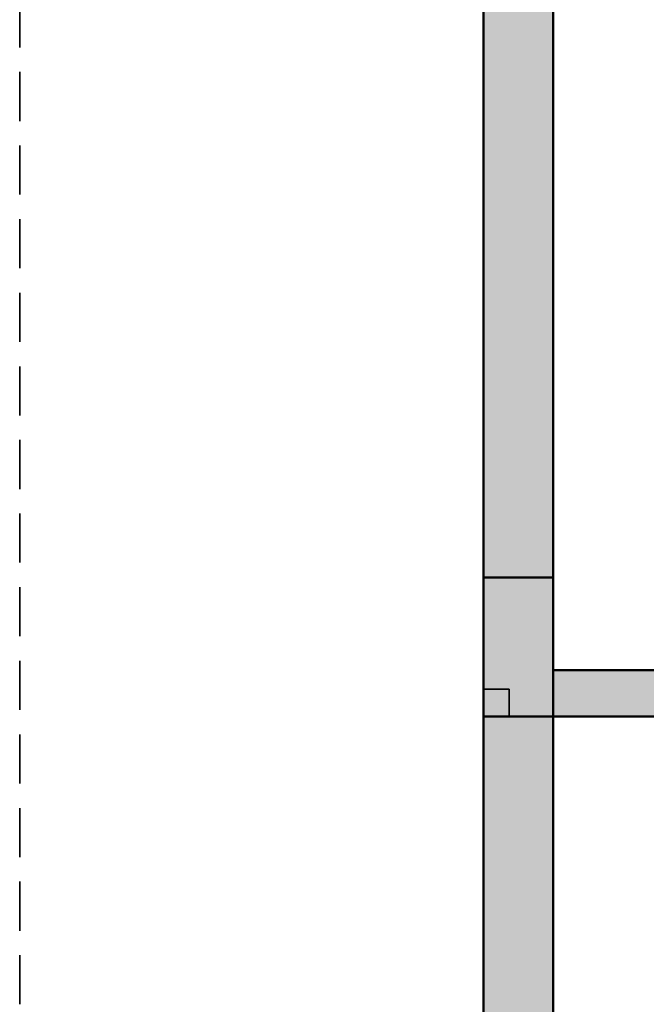
# Model space of a CAD drawing. Units: inches. Extents: x -7 to 1228, y -146 to 1091.
# Tile 43 of 88: x 0 to 81, y 531 to 658. Entities that reach past the tile are written whole.
import ezdxf

# ---------------------------------------------------------------- set-up
doc = ezdxf.new("R2010")
doc.units = ezdxf.units.IN
doc.linetypes.add('DASHED2', pattern=[9.525, 6.35, -3.175])
for name, color, linetype, lineweight in [('A-COLS', 6, 'Continuous', 35), ('A-WALL', 7, 'Continuous', 50), ('A-WALL-PATT', 251, 'Continuous', 13), ('C-PROP', 1, 'DASHED2', 35)]:
    doc.layers.add(name, color=color, linetype=linetype, lineweight=lineweight)

msp = doc.modelspace()

# ---------------------------------------------------------------- hatches: boundary and pattern name
at = {"layer": 'A-COLS'}
h = msp.add_hatch(color=256, dxfattribs=at)
h.dxf.hatch_style = 1
h.paths.add_polyline_path([(69, 586), (60, 586), (60, 571.55), (63.29, 571.55), (63.29, 568), (69, 568)])
h = msp.add_hatch(color=256, dxfattribs=at)
h.dxf.hatch_style = 1
h.paths.add_polyline_path([(63.29, 571.55), (60, 571.55), (60, 568), (63.29, 568)])
at = {"layer": 'A-WALL-PATT'}
h = msp.add_hatch(color=256, dxfattribs=at)
h.dxf.hatch_style = 1
h.paths.add_polyline_path([(69, 568), (60, 568), (60, 493), (63.29, 493), (69, 493)])
h.paths.add_polyline_path([(69, 662.41), (60, 662.41), (60, 586), (69, 586)], flags=17)
h.paths.add_polyline_path([(69, 723), (184, 723), (184, 734), (179, 734), (179, 728), (69, 728), (69, 741.62), (60, 741.62), (60, 698.41), (69, 698.41)], flags=17)
h.paths.add_polyline_path([(69, 782), (231, 782), (231, 728), (231, 723), (231, 586), (236, 586), (236, 787), (69, 787), (69, 800.13), (60, 800.13), (60, 765.62), (69, 765.62)])
h.paths.add_polyline_path([(184, 842), (189, 842), (189, 848), (173, 848), (173, 842), (179, 842), (179, 787), (184, 787)])
h.paths.add_polyline_path([(118.22, 69), (69, 69), (69, 60), (118.22, 60)])
h.paths.add_polyline_path([(227, 69), (154.22, 69), (154.22, 60), (227, 60)])
h.paths.add_polyline_path([(236, 60), (232.71, 60), (227, 60), (227, 36), (236, 36)])
h.paths.add_polyline_path([(389, 60), (380, 60), (380, 36), (389, 36)])
h.paths.add_polyline_path([(384, 181), (380, 181), (380, 115), (380, 78), (384, 78)])
h.paths.add_polyline_path([(380, 115), (334.55, 115), (334.55, 109), (380, 109)])
h.paths.add_polyline_path([(274.55, 115), (236, 115), (236, 201), (232.71, 201), (231, 201), (231, 78), (236, 78), (236, 109), (274.55, 109)])
h.paths.add_polyline_path([(69, 123), (60, 123), (60, 78), (69, 78)])
h.paths.add_polyline_path([(69, 201), (60, 201), (60, 159), (69, 159)])
h.paths.add_polyline_path([(143, 219), (69, 219), (69, 213), (143, 213)], flags=17)
h.paths.add_polyline_path([(189, 219), (184, 219), (184, 274), (231, 274), (231, 219), (236, 219), (236, 279), (184, 279), (184, 297), (179, 297), (179, 279), (69, 279), (69, 290.91), (60, 290.91), (60, 262.18), (69, 262.18), (69, 274), (179, 274), (179, 219), (173, 219), (173, 213), (189, 213)])
h.paths.add_polyline_path([(69, 238.18), (60, 238.18), (60, 219), (69, 219)], flags=17)
h.paths.add_polyline_path([(69, 333), (60, 333), (60, 314.91), (69, 314.91), (69, 316.96)])
h.paths.add_polyline_path([(190, 338), (184, 338), (69, 338), (69, 333), (179, 333), (179, 327), (184, 327), (184, 333.02), (190, 333.05)])
h.paths.add_polyline_path([(69, 386.81), (60, 386.81), (60, 351), (69, 351)])
h.paths.add_polyline_path([(69, 475), (60, 475), (60, 422.81), (69, 422.81)])
h.paths.add_polyline_path([(236, 475), (231, 475), (231, 351.24), (236, 351.24)])
h.paths.add_polyline_path([(384, 475), (380, 475), (380, 362), (384, 362)])
h.paths.add_polyline_path([(547, 307), (439, 307), (439, 356), (445, 356), (445, 362), (433, 362), (433, 307), (380, 307), (380, 244), (380, 241), (384, 241), (384, 301), (433, 301), (433, 277), (439, 277), (439, 301), (547, 301)])
h.paths.add_polyline_path([(547, 241), (439, 241), (439, 247), (433, 247), (433, 235), (547, 235)])
h.paths.add_polyline_path([(450, 69), (440.29, 69), (424.89, 69), (389, 69), (389, 60), (450, 60)])
h.paths.add_polyline_path([(547, 69), (486, 69), (486, 60), (547, 60)])
h.paths.add_polyline_path([(556, 148.27), (547, 148.27), (547, 78), (556, 78)])
h.paths.add_polyline_path([(556, 223), (547, 223), (547, 195), (547, 184.27), (556, 184.27)])
h.paths.add_polyline_path([(556, 311.19), (547, 311.19), (547, 273.08), (556, 273.08)])
h.paths.add_polyline_path([(556, 344), (552.71, 344), (547, 344), (547, 335.19), (556, 335.19)])
h.paths.add_polyline_path([(556, 249.08), (547, 249.08), (547, 241), (556, 241)])
h.paths.add_polyline_path([(547, 362), (475, 362), (475, 356), (547, 356)], flags=0)
h.paths.add_polyline_path([(556, 399.62), (547, 399.62), (547, 362), (556, 362)])
h.paths.add_polyline_path([(556, 475), (547, 475), (547, 435.62), (556, 435.62)])
h.paths.add_polyline_path([(547, 493), (389, 493), (389, 487), (547, 487)])
h.paths.add_polyline_path([(380, 493), (278, 493), (278, 487), (380, 487)])
h.paths.add_polyline_path([(227, 493), (69, 493), (69, 487), (227, 487)])
h.paths.add_polyline_path([(643, 122.44), (634, 122.44), (634, 78), (643, 78)])
h.paths.add_polyline_path([(702.5, 69), (692.79, 69), (677.39, 69), (643, 69), (643, 60), (702.5, 60)])
h.paths.add_polyline_path([(798, 69), (738.5, 69), (738.5, 60), (798, 60)])
h.paths.add_polyline_path([(807, 60), (803.71, 60), (798, 60), (798, 36), (807, 36)])
h.paths.add_polyline_path([(807, 109), (846.75, 109), (846.75, 115), (807, 115), (807, 159), (802, 159), (802, 78), (807, 78)])
h.paths.add_polyline_path([(807, 201), (802, 201), (802, 195), (807, 195)])
h.paths.add_polyline_path([(643, 201), (634, 201), (634, 158.44), (643, 158.44)])
h.paths.add_polyline_path([(756, 225), (751, 225), (751, 219), (643, 219), (643, 213), (756, 213)])
h.paths.add_polyline_path([(643, 240.85), (634, 240.85), (634, 219), (643, 219)])
h.paths.add_polyline_path([(643, 274), (643, 288.63), (634, 288.63), (634, 264.85), (643, 264.85)])
h.paths.add_polyline_path([(802, 279), (756, 279), (756, 297), (751, 297), (751, 279), (643, 279), (643, 274), (751, 274), (751, 255), (756, 255), (756, 274), (802, 274)])
h.paths.add_polyline_path([(807, 333), (803.71, 333), (802, 333), (802, 279), (802, 274), (802, 219), (807, 219)])
h.paths.add_polyline_path([(956, 182), (951, 182), (951, 115), (906.75, 115), (906.75, 109), (951, 109), (951, 78), (956, 78)])
h.paths.add_polyline_path([(960, 60), (951, 60), (951, 36), (960, 36)])
h.paths.add_polyline_path([(1021, 69), (1005.78, 69), (960, 69), (960, 60), (1021, 60)])
h.paths.add_polyline_path([(956, 224), (951, 224), (951, 218), (956, 218)])
h.paths.add_polyline_path([(956, 302), (1004, 302), (1004, 278), (1010, 278), (1010, 302), (1118, 302), (1118, 290.81), (1127, 290.81), (1127, 326.97), (1118, 326.97), (1118, 320.97), (1118, 307), (1010, 307), (1010, 356), (1016, 356), (1016, 362), (1004, 362), (1004, 307), (951, 307), (951, 244), (951, 242), (954.29, 242), (956, 242)])
h.paths.add_polyline_path([(643, 333), (634, 333), (634, 312.63), (643, 312.63), (643, 316.96)])
h.paths.add_polyline_path([(756, 338), (643, 338), (643, 333), (751, 333), (751, 327), (756, 327)])
h.paths.add_polyline_path([(643, 388), (634, 388), (634, 351), (643, 351)])
h.paths.add_polyline_path([(807, 357), (802, 357), (802, 351), (807, 351)])
h.paths.add_polyline_path([(807, 475), (802, 475), (802, 393), (807, 393)])
h.paths.add_polyline_path([(643, 475), (634, 475), (634, 424), (643, 424)])
h.paths.add_polyline_path([(798, 493), (643, 493), (643, 487), (798, 487)])
h.paths.add_polyline_path([(634, 493), (556, 493), (556, 487), (634, 487)])
h.paths.add_polyline_path([(813, 493), (807, 493), (807, 487), (813, 487)])
h.paths.add_polyline_path([(951, 493), (849, 493), (849, 487), (951, 487)])
h.paths.add_polyline_path([(956, 484), (951, 484), (951, 374), (956, 374)])
h.paths.add_polyline_path([(1109, 493), (969, 493), (969, 487), (1109, 487)])
h.paths.add_polyline_path([(1127, 484), (1118, 484), (1118, 450.64), (1127, 450.64)])
h.paths.add_polyline_path([(1127, 414.64), (1118, 414.64), (1118, 365), (1127, 365)])
h.paths.add_polyline_path([(1109, 362), (1046, 362), (1046, 356), (1109, 356)], flags=17)
h.paths.add_polyline_path([(1127, 356), (1123.45, 356), (1118, 356), (1118, 350.97), (1127, 350.97)], flags=0)
h.paths.add_polyline_path([(1127, 266.81), (1118, 266.81), (1118, 262.36), (1118, 242), (1127, 242)], flags=17)
h.paths.add_polyline_path([(1118, 242), (1010, 242), (1010, 248), (1004, 248), (1004, 237), (1118, 237)])
h.paths.add_polyline_path([(1127, 224), (1118, 224), (1118, 170), (1127, 170)])
h.paths.add_polyline_path([(1127, 134), (1118, 134), (1118, 78), (1127, 78)])
h.paths.add_polyline_path([(1118, 69), (1057, 69), (1057, 60), (1118, 60)])
h.paths.add_polyline_path([(227, 571.55), (227, 574), (69, 574), (69, 568), (227, 568)])
h.paths.add_polyline_path([(380, 571.55), (380, 574), (278, 574), (278, 568), (380, 568)])
h.paths.add_polyline_path([(242, 574), (236, 574), (236, 568), (242, 568)])
h.paths.add_polyline_path([(547, 571.55), (547, 574), (389, 574), (389, 568), (547, 568)])
h.paths.add_polyline_path([(384, 733), (380, 733), (380, 586), (384, 586)])
h.paths.add_polyline_path([(556, 646), (634, 646), (634, 655), (547, 655), (547, 586), (556, 586)])
h.paths.add_polyline_path([(634, 574), (556, 574), (556, 568), (634, 568)])
h.paths.add_polyline_path([(643, 655), (634, 655), (634, 586), (643, 586)])
h.paths.add_polyline_path([(798, 574), (643, 574), (643, 568), (798, 568)])
h.paths.add_polyline_path([(643, 663.85), (634, 663.85), (634, 655), (643, 655)])
h.paths.add_polyline_path([(556, 676.97), (547, 676.97), (547, 655), (556, 655)])
h.paths.add_polyline_path([(556, 733), (547, 733), (547, 712.97), (556, 712.97)])
h.paths.add_polyline_path([(643, 710), (634, 710), (634, 699.85), (643, 699.85)])
h.paths.add_polyline_path([(807, 668), (802, 668), (802, 586), (807, 586)])
h.paths.add_polyline_path([(951, 574), (849, 574), (849, 568), (951, 568)])
h.paths.add_polyline_path([(956, 691), (951, 691), (951, 577), (956, 577)])
h.paths.add_polyline_path([(1109, 574), (969, 574), (969, 568), (1109, 568)])
h.paths.add_polyline_path([(1127, 643.4), (1118, 643.4), (1118, 577), (1127, 577)])
h.paths.add_polyline_path([(1127, 568), (1123.45, 568), (1118, 568), (1118, 493), (1127, 493)])
h.paths.add_polyline_path([(1127, 733), (1118, 733), (1118, 679.4), (1127, 679.4)])
h.paths.add_polyline_path([(1127, 777.35), (1118, 777.35), (1118, 770.04), (1118, 751), (1127, 751)], flags=17)
h.paths.add_polyline_path([(1118, 751), (1010, 751), (1010, 757), (1004, 757), (1004, 745), (1118, 745)])
h.paths.add_polyline_path([(956, 811), (1004, 811), (1004, 787), (1010, 787), (1010, 811), (1017.87, 811), (1017.87, 811.63, -0.414214), (1018.25, 812), (1031.98, 812, -0.414214), (1032.35, 811.63), (1032.35, 811), (1118, 811), (1118, 801.35), (1127, 801.35), (1127, 834.69), (1118, 834.69), (1118, 830.24), (1118, 817), (1010, 817), (1010, 866), (1016, 866), (1016, 872), (1004, 872), (1004, 817), (956, 817), (956, 866), (951, 866), (951, 751), (954.29, 751), (956, 751)])
h.paths.add_polyline_path([(1118, 872), (1046, 872), (1046, 866), (1118, 866)], flags=17)
h.paths.add_polyline_path([(1127, 924.71), (1118, 924.71), (1118, 884), (1127, 884)])
h.paths.add_polyline_path([(1127, 866), (1123.71, 866), (1118, 866), (1118, 858.69), (1127, 858.69)], flags=17)
h.paths.add_polyline_path([(956, 983), (951, 983), (951, 952), (807, 952), (807, 983), (802, 983), (802, 902), (807, 902), (807, 946), (951, 946), (951, 884), (956, 884)])
h.paths.add_polyline_path([(807, 842), (802, 842), (802, 787), (756, 787), (756, 806), (751, 806), (751, 787), (643, 787), (643, 782), (751, 782), (751, 764), (756, 764), (756, 782), (802, 782), (802, 728), (807, 728)])
h.paths.add_polyline_path([(756, 848), (643, 848), (643, 842), (751, 842), (751, 836), (756, 836)])
h.paths.add_polyline_path([(756, 734), (751, 734), (751, 728), (643, 728), (643, 723), (756, 723)])
h.paths.add_polyline_path([(643, 749.79), (634, 749.79), (634, 728), (637.29, 728), (643, 728)])
h.paths.add_polyline_path([(643, 805.41), (634, 805.41), (634, 773.79), (643, 773.79)])
h.paths.add_polyline_path([(643, 896.66), (634, 896.66), (634, 860), (637.29, 860), (643, 860)])
h.paths.add_polyline_path([(643, 842), (634, 842), (634, 829.41), (643, 829.41)])
h.paths.add_polyline_path([(643, 983), (634, 983), (634, 932.66), (643, 932.66)])
h.paths.add_polyline_path([(1127, 983), (1118, 983), (1118, 960.71), (1127, 960.71)])
h.paths.add_polyline_path([(1118, 1001), (1077.53, 1001), (1077.53, 992), (1118, 992)])
h.paths.add_polyline_path([(1041.53, 1001), (960, 1001), (960, 992), (1041.53, 992)])
h.paths.add_polyline_path([(960, 1025), (951, 1025), (951, 1001), (954.29, 1001), (960, 1001)])
h.paths.add_polyline_path([(807, 1025), (798, 1025), (798, 1001), (807, 1001)])
h.paths.add_polyline_path([(798, 1001), (738.5, 1001), (738.5, 992), (798, 992)])
h.paths.add_polyline_path([(702.5, 1001), (643, 1001), (643, 992), (702.5, 992)])
h.paths.add_polyline_path([(547, 1001), (499.11, 1001), (499.11, 992), (547, 992)])
h.paths.add_polyline_path([(463.11, 1001), (389, 1001), (389, 992), (463.11, 992)])
h.paths.add_polyline_path([(389, 1025), (380, 1025), (380, 1022), (380, 1001), (383.29, 1001), (389, 1001)])
h.paths.add_polyline_path([(236, 1025), (227, 1025), (227, 1001), (236, 1001)])
h.paths.add_polyline_path([(236, 983), (231, 983), (231, 860), (236, 860)])
h.paths.add_polyline_path([(274.55, 952), (236, 952), (236, 946), (274.55, 946)])
h.paths.add_polyline_path([(380, 952), (334.55, 952), (334.55, 946), (380, 946)])
h.paths.add_polyline_path([(384, 983), (380, 983), (380, 884), (383.29, 884), (384, 884)])
h.paths.add_polyline_path([(227, 1001), (155.01, 1001), (155.01, 992), (162.87, 992), (227, 992)])
h.paths.add_polyline_path([(119.01, 1001), (69, 1001), (69, 992), (119.01, 992)])
h.paths.add_polyline_path([(69, 983), (60, 983), (60, 922.99), (69, 922.99)])
h.paths.add_polyline_path([(69, 886.99), (60, 886.99), (60, 860), (63.29, 860), (69, 860)])
h.paths.add_polyline_path([(143, 848), (69, 848), (69, 842), (143, 842)])

# ---------------------------------------------------------------- linework, layer by layer
at = {"layer": 'A-COLS'}
msp.add_lwpolyline([(60, 568), (63.29, 568), (63.29, 571.55), (60, 571.55)], close=True, dxfattribs=at)
at = {"layer": 'A-WALL'}
for p, q in [((60, 1001), (60, 60)), ((69, 723), (69, 574)), ((69, 586), (60, 586)), ((60, 586), (60, 568)), ((69, 568), (69, 586)), ((231, 574), (69, 574)), ((231, 568), (60, 568)), ((60, 568), (69, 568)), ((69, 568), (69, 279))]:
    msp.add_line(p, q, dxfattribs=at)
at = {"layer": 'C-PROP'}
msp.add_line((0, 1061), (0, 0), dxfattribs=at)

doc.saveas('drawing.dxf')
